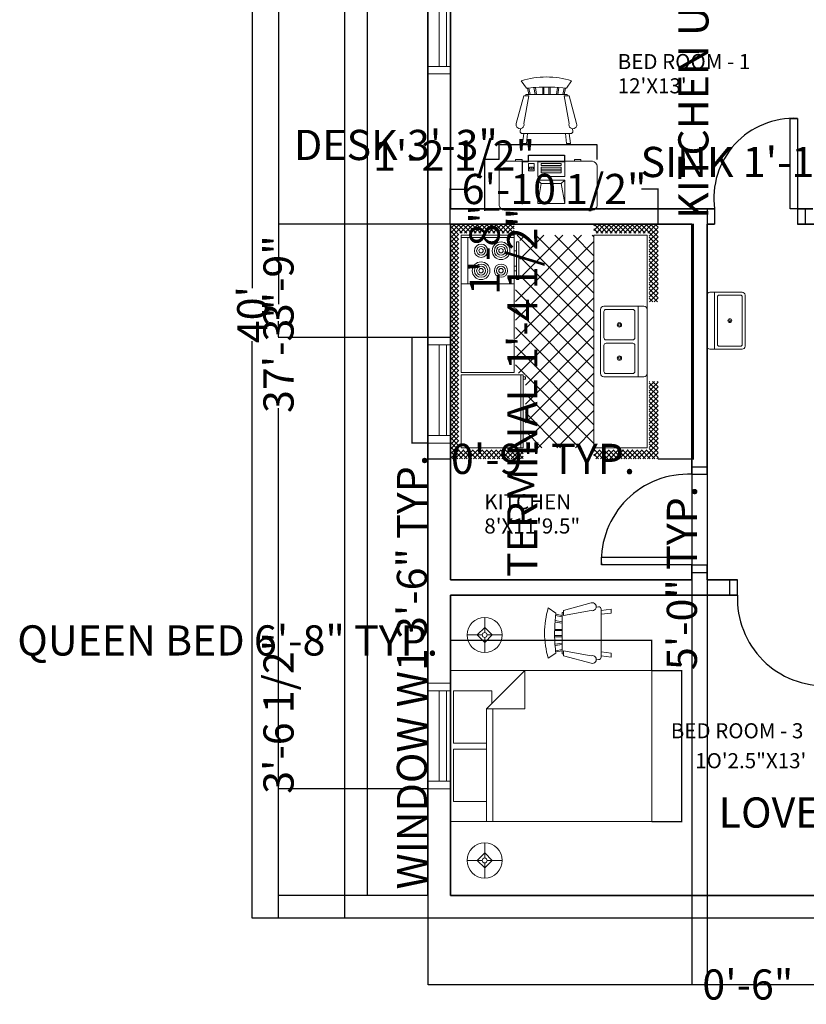
# Model space of a CAD drawing. Units: inches. Extents: x -107 to 531, y -526 to 131.
# Tile 1 of 4: x -107 to 205, y -506 to -114. Entities that reach past the tile are written whole.
import ezdxf

# ---------------------------------------------------------------- set-up
doc = ezdxf.new("R2010")
doc.units = ezdxf.units.IN
doc.header["$MEASUREMENT"] = 0
for name, color, linetype, lineweight in [('A-ANNO-DIMS', 2, 'Continuous', 18), ('A-AREA-IDEN', 7, 'Continuous', 25), ('A-DOOR', 3, 'Continuous', 25), ('A-EQPM', 9, 'Continuous', 18), ('A-FLOR-FIXT', 9, 'Continuous', 18), ('A-FURN', 8, 'Continuous', 18), ('A-GLAZ', 4, 'Continuous', 18), ('A-WALL', 7, 'Continuous', 35), ('C-PROP', 8, 'Continuous', 25)]:
    doc.layers.add(name, color=color, linetype=linetype, lineweight=lineweight)
doc.styles.get("Standard").update_dxf_attribs({"font": 'arial.ttf'})
doc.dimstyles.get("Standard").update_dxf_attribs({"dimtxt": 12, "dimasz": 0.18, "dimexe": 0.18, "dimexo": 0.0625, "dimgap": 0.09, "dimtad": 0, "dimdec": 1, "dimzin": 0, "dimdsep": 46, "dimlunit": 3, "dimtxsty": 'Standard', "dimcen": 0.09, "dimadec": 0, "dimazin": 0, "dimtfac": 1, "dimtdec": 1, "dimtofl": 0, "dimtmove": 0, "dimatfit": 3, "dimfxl": 1, "dimtolj": 1, "dimtzin": 0, "dimarcsym": 0})

# ---------------------------------------------------------------- blocks, each defined once
blk = doc.blocks.new('Bed - Queen')
for p, q in [((0, -80.00003), (0, 0)), ((0, 0), (59.99999, 0)), ((59.99999, 0), (59.99999, -80.00003)), ((7.99999, -1.2), (28.79998, -1.2)), ((7.99999, -14.4), (7.99999, -1.2)), ((28.79998, -1.2), (28.79998, -14.4)), ((31.19999, -1.2), (51.99999, -1.2)), ((31.19999, -14.4), (31.19999, -1.2)), ((51.99999, -1.2), (51.99999, -16.4)), ((0, -14.4), (44.8, -14.4)), ((59.99999, -29.6), (44.8, -14.4)), ((44.8, -14.4), (44.8, -29.6)), ((44.8, -16.8), (0, -16.8)), ((51.99999, -16.4), (46.79936, -16.4)), ((44.8, -29.6), (59.99999, -29.6)), ((59.99999, -80.00003), (0, -80.00003))]:
    blk.add_line(p, q)
blk = doc.blocks.new('Kitchen Layout - 7 x 8 ft')
for p, q in [((-5, 81.32), (2.68, 89)), ((-5, 83.44), (0.56, 89)), ((-5, 85.56), (-1.56, 89)), ((-5, 87.68), (-3.68, 89)), ((1.09, 85), (-2.91, 89)), ((3.21, 85), (-0.79, 89)), ((0.81, 85), (4.81, 89)), ((5.34, 85), (1.34, 89)), ((2.93, 85), (6.93, 89)), ((7.46, 85), (3.46, 89)), ((5.05, 85), (9.05, 89)), ((9.58, 85), (5.58, 89)), ((7.17, 85), (11.17, 89)), ((11.7, 85), (7.7, 89)), ((9.29, 85), (13.29, 89)), ((13.82, 85), (9.82, 89)), ((11.41, 85), (15.41, 89)), ((15.94, 85), (11.94, 89)), ((13.53, 85), (17.53, 89)), ((18.06, 85), (14.06, 89)), ((15.65, 85), (19.65, 89)), ((20.18, 85), (16.18, 89)), ((17.78, 85), (21.78, 89)), ((22.31, 85), (18.31, 89)), ((19.9, 85), (23.9, 89)), ((24.43, 85), (20.43, 89)), ((22.02, 85), (26.02, 89)), ((26.55, 85), (22.55, 89)), ((24.14, 85), (28.14, 89)), ((28.67, 85), (24.67, 89)), ((26.26, 85), (30.26, 89)), ((30.79, 85), (26.79, 89)), ((28.38, 85), (32.38, 89)), ((32.91, 85), (28.91, 89)), ((30.5, 85), (34.5, 89)), ((35.03, 85), (31.03, 89)), ((32.63, 85), (36.63, 89)), ((37.16, 85), (33.16, 89)), ((34.75, 85), (38.75, 89)), ((39.28, 85), (35.28, 89)), ((36.87, 85), (40.87, 89)), ((41.4, 85), (37.4, 89)), ((38.99, 85), (42.99, 89)), ((43.52, 85), (39.52, 89)), ((41.11, 85), (45.11, 89)), ((45.64, 85), (41.64, 89)), ((43.23, 85), (47.23, 89)), ((47.76, 85), (43.76, 89)), ((45.35, 85), (49.35, 89)), ((49.88, 85), (45.88, 89)), ((47.47, 85), (51.47, 89)), ((52, 85), (48, 89)), ((49.6, 85), (53.6, 89)), ((54.13, 85), (50.13, 89)), ((51.72, 85), (55.72, 89)), ((56.25, 85), (52.25, 89)), ((53.84, 85), (57.84, 89)), ((58.37, 85), (54.37, 89)), ((55.96, 85), (59.96, 89)), ((60.49, 85), (56.49, 89)), ((58.08, 85), (62.08, 89)), ((62.61, 85), (58.61, 89)), ((60.2, 85), (64.2, 89)), ((64.73, 85), (60.73, 89)), ((62.32, 85), (66.32, 89)), ((66.85, 85), (62.85, 89)), ((64.45, 85), (68.45, 89)), ((68.97, 85), (64.97, 89)), ((66.57, 85), (70.57, 89)), ((71.1, 85), (67.1, 89)), ((68.69, 85), (72.69, 89)), ((73.22, 85), (69.22, 89)), ((70.81, 85), (74.81, 89)), ((75.34, 85), (71.34, 89)), ((72.93, 85), (76.93, 89)), ((77.46, 85), (73.46, 89)), ((75.05, 85), (79.05, 89)), ((79.58, 85), (75.58, 89)), ((77.17, 85), (81.17, 89)), ((81.7, 85), (77.7, 89)), ((79.29, 85), (83.29, 89)), ((83.82, 85), (79.82, 89)), ((81.42, 85), (85.42, 89)), ((85.95, 85), (81.95, 89)), ((83.54, 85), (87.54, 89)), ((88.07, 85), (84.07, 89)), ((85.66, 85), (89.66, 89)), ((90.19, 85), (86.19, 89)), ((87.78, 85), (91.78, 89)), ((92.31, 85), (88.31, 89)), ((89.9, 85), (93.9, 89)), ((94.43, 85), (90.43, 89)), ((92.02, 85), (96.02, 89)), ((96.55, 85), (92.55, 89)), ((94.14, 85), (98.14, 89)), ((101, 82.67), (94.67, 89)), ((96.27, 85), (100.27, 89)), ((101, 84.79), (96.79, 89)), ((101, 86.92), (98.92, 89)), ((-1, 84.97), (-5, 88.97)), ((-1, 82.85), (-5, 86.85)), ((-1, 80.73), (-5, 84.73)), ((97, 83.61), (101, 87.61)), ((97, 81.49), (101, 85.49)), ((101, 80.55), (97, 84.55)), ((-5, 79.19), (-1, 83.19)), ((-1, 78.61), (-5, 82.61)), ((-5, 77.07), (-1, 81.07)), ((-1, 76.49), (-5, 80.49)), ((34, 84), (96, 84)), ((34, 60), (34, 84)), ((74, 81), (95, 81)), ((96, 84), (96, 60)), ((97, 79.37), (101, 83.37)), ((101, 78.43), (97, 82.43)), ((97, 77.25), (101, 81.25)), ((101, 76.31), (97, 80.31)), ((-5, 74.95), (-1, 78.95)), ((-1, 74.36), (-5, 78.36)), ((-5, 72.83), (-1, 76.83)), ((-1, 72.24), (-5, 76.24)), ((97, 75.13), (101, 79.13)), ((101, 74.19), (97, 78.19)), ((97, 73.01), (101, 77.01)), ((101, 72.07), (97, 76.07)), ((-5, 70.71), (-1, 74.71)), ((-1, 70.12), (-5, 74.12)), ((-5, 68.59), (-1, 72.59)), ((-1, 68), (-5, 72)), ((97, 70.89), (101, 74.89)), ((101, 69.95), (97, 73.95)), ((97, 68.76), (101, 72.76)), ((101, 67.82), (97, 71.82)), ((-5, 66.47), (-1, 70.47)), ((-1, 65.88), (-5, 69.88)), ((-5, 64.35), (-1, 68.35)), ((-1, 63.76), (-5, 67.76)), ((97, 66.64), (101, 70.64)), ((101, 65.7), (97, 69.7)), ((97, 64.52), (101, 68.52)), ((101, 63.58), (97, 67.58)), ((-5, 62.22), (-1, 66.22)), ((-1, 61.64), (-5, 65.64)), ((-5, 60.1), (-1, 64.1)), ((-1, 59.52), (-5, 63.52)), ((97, 62.4), (101, 66.4)), ((101, 61.46), (97, 65.46)), ((97, 60.28), (101, 64.28)), ((100.34, 60), (97, 63.34)), ((-5, 57.98), (-1, 61.98)), ((-1, 57.39), (-5, 61.39)), ((-1.73, 56), (-5, 59.27)), ((-4.86, 56), (-1, 59.86)), ((10.4, 24), (45.9, 59.5)), ((18.88, 24), (54.38, 59.5)), ((27.37, 24), (62.87, 59.5)), ((33.03, 55.11), (37.41, 59.5)), ((67.71, 24), (33.68, 58.04)), ((96, 60), (34, 60)), ((35.85, 24), (71.35, 59.5)), ((76.2, 24), (40.7, 59.5)), ((84.68, 24), (49.18, 59.5)), ((93.17, 24), (57.67, 59.5)), ((61.31, 24), (96, 58.69)), ((96, 29.65), (66.15, 59.5)), ((80, 60), (80, 59)), ((82, 59), (82, 60)), ((87, 59), (87, 60)), ((89, 60), (89, 59)), ((98.22, 60), (97, 61.22)), ((98.84, 60), (101, 62.16)), ((100.96, 60), (101, 60.04)), ((-3.85, 56), (-5, 57.15)), ((-2.74, 56), (-1, 57.74)), ((0, 57), (33, 57)), ((0, 30.57), (24.43, 55)), ((0, 39.06), (15.94, 55)), ((0, 47.54), (7.46, 55)), ((1.91, 24), (32.91, 55)), ((33.77, 24), (2.77, 55)), ((42.26, 24), (11.26, 55)), ((50.74, 24), (19.74, 55)), ((59.23, 24), (28.23, 55)), ((31, 55), (31, 56)), ((32, 55), (31, 55)), ((32, 56), (32, 55)), ((44.34, 24), (77.84, 57.5)), ((52.82, 24), (86.32, 57.5)), ((96, 38.14), (76.64, 57.5)), ((96, 46.63), (85.13, 57.5)), ((96, 55.11), (93.57, 57.54)), ((25.29, 24), (0, 49.29)), ((69.79, 24), (96, 50.21)), ((16.8, 24), (0, 40.8)), ((78.28, 24), (96, 41.72)), ((8.32, 24), (0, 32.32)), ((86.76, 24), (96, 33.24)), ((-5, 21.92), (-2.92, 24)), ((-5, 19.8), (-1, 23.8)), ((-1, 19.21), (-5, 23.21)), ((-1, 21.33), (-3.67, 24)), ((-1, 23.45), (-1.55, 24)), ((0, 24), (96, 24)), ((0, 0), (0, 24)), ((95.25, 24), (96, 24.75)), ((96, 24), (96, 0)), ((97, 22.1), (98.9, 24)), ((97, 19.97), (101, 23.97)), ((101, 19.03), (97, 23.03)), ((101, 21.16), (98.16, 24)), ((101, 23.28), (100.28, 24)), ((-5, 17.68), (-1, 21.68)), ((-1, 17.09), (-5, 21.09)), ((-5, 15.55), (-1, 19.55)), ((-1, 14.97), (-5, 18.97)), ((47.25, 6.5), (47.25, 18.5)), ((48.75, 18.5), (48.75, 6.5)), ((97, 17.85), (101, 21.85)), ((101, 16.91), (97, 20.91)), ((97, 15.73), (101, 19.73)), ((101, 14.79), (97, 18.79)), ((-5, 13.43), (-1, 17.43)), ((-1, 12.85), (-5, 16.85)), ((-5, 11.31), (-1, 15.31)), ((-1, 10.73), (-5, 14.73)), ((97, 13.61), (101, 17.61)), ((101, 12.67), (97, 16.67)), ((97, 11.49), (101, 15.49)), ((101, 10.55), (97, 14.55)), ((97, 9.37), (101, 13.37)), ((-5, 9.19), (-1, 13.19)), ((-1, 8.6), (-5, 12.6)), ((-5, 7.07), (-1, 11.07)), ((-1, 6.48), (-5, 10.48)), ((-5, 4.95), (-1, 8.95)), ((101, 8.43), (97, 12.43)), ((97, 7.25), (101, 11.25)), ((101, 6.31), (97, 10.31)), ((97, 5.12), (101, 9.12)), ((-1, 4.36), (-5, 8.36)), ((-5, 2.83), (-1, 6.83)), ((-1, 2.24), (-5, 6.24)), ((-5, 0.71), (-1, 4.71)), ((101, 4.18), (97, 8.18)), ((97, 3), (101, 7)), ((101, 2.06), (97, 6.06)), ((97, 0.88), (101, 4.88)), ((-1, 0.12), (-5, 4.12)), ((-5, -1.42), (-1, 2.58)), ((2, -5), (-5, 2)), ((-5, -3.54), (-1, 0.46)), ((96, 0), (0, 0)), ((64, 4), (32, 4)), ((93.24, -5), (101, 2.76)), ((95.36, -5), (101, 0.64)), ((101, -0.06), (97, 3.94)), ((101, -2.18), (97, 1.82)), ((-0.12, -5), (-5, -0.12)), ((-2.25, -5), (-5, -2.25)), ((-4.37, -5), (-5, -4.37)), ((-4.34, -5), (-0.34, -1)), ((-2.22, -5), (1.78, -1)), ((-0.1, -5), (3.9, -1)), ((4.12, -5), (0.12, -1)), ((2.02, -5), (6.02, -1)), ((6.24, -5), (2.24, -1)), ((4.14, -5), (8.14, -1)), ((8.36, -5), (4.36, -1)), ((6.27, -5), (10.27, -1)), ((10.48, -5), (6.48, -1)), ((8.39, -5), (12.39, -1)), ((12.6, -5), (8.6, -1)), ((10.51, -5), (14.51, -1)), ((14.73, -5), (10.73, -1)), ((12.63, -5), (16.63, -1)), ((16.85, -5), (12.85, -1)), ((14.75, -5), (18.75, -1)), ((18.97, -5), (14.97, -1)), ((16.87, -5), (20.87, -1)), ((21.09, -5), (17.09, -1)), ((18.99, -5), (22.99, -1)), ((23.21, -5), (19.21, -1)), ((21.11, -5), (25.11, -1)), ((25.33, -5), (21.33, -1)), ((23.24, -5), (27.24, -1)), ((27.45, -5), (23.45, -1)), ((25.36, -5), (29.36, -1)), ((29.57, -5), (25.57, -1)), ((27.48, -5), (30, -2.48)), ((30, -3.3), (27.7, -1)), ((30, -1.18), (29.82, -1)), ((66, -2.54), (67.54, -1)), ((66, -4.66), (69.66, -1)), ((69.88, -5), (66, -1.12)), ((67.76, -5), (66, -3.24)), ((67.78, -5), (71.78, -1)), ((72, -5), (68, -1)), ((69.9, -5), (73.9, -1)), ((74.12, -5), (70.12, -1)), ((72.03, -5), (76.03, -1)), ((76.24, -5), (72.24, -1)), ((74.15, -5), (78.15, -1)), ((78.36, -5), (74.36, -1)), ((76.27, -5), (80.27, -1)), ((80.49, -5), (76.49, -1)), ((78.39, -5), (82.39, -1)), ((82.61, -5), (78.61, -1)), ((80.51, -5), (84.51, -1)), ((84.73, -5), (80.73, -1)), ((82.63, -5), (86.63, -1)), ((86.85, -5), (82.85, -1)), ((84.75, -5), (88.75, -1)), ((88.97, -5), (84.97, -1)), ((86.88, -5), (90.88, -1)), ((91.09, -5), (87.09, -1)), ((89, -5), (93, -1)), ((93.21, -5), (89.21, -1)), ((91.12, -5), (95.12, -1)), ((95.34, -5), (91.34, -1)), ((97.46, -5), (93.46, -1)), ((99.58, -5), (95.58, -1)), ((101, -4.3), (97, -0.3)), ((97.48, -5), (101, -1.48)), ((99.6, -5), (101, -3.6)), ((29.6, -5), (30, -4.6))]:
    blk.add_line(p, q)
for points in [[(0, 56), (0, 84), (33, 84), (33, 56)], [(74, 60), (74, 84), (95, 84), (95, 60)], [(76, 58), (76, 59), (93, 59), (93, 58)]]:
    blk.add_lwpolyline(points, close=True)
for points in [[(32, 1.5), (32, 19.5)], [(33.5, 21), (62.5, 21)], [(33.5, 6.5), (33.5, 18.5)], [(34.5, 19.5), (46.25, 19.5)], [(49.75, 19.5), (61.5, 19.5)], [(62.5, 18.5), (62.5, 6.5)], [(64, 19.5), (64, 1.5)], [(46.25, 5.5), (34.5, 5.5)], [(61.5, 5.5), (49.75, 5.5)], [(62.5, 0), (33.5, 0)]]:
    blk.add_lwpolyline(points)
for centre, radius in [((80, 75), 4), ((80, 75), 3), ((80, 75), 2), ((80, 75), 1), ((89, 75), 3), ((89, 75), 2), ((89, 75), 1), ((80, 66), 3), ((80, 66), 2), ((80, 66), 1), ((89, 66), 4), ((89, 66), 3), ((89, 66), 2), ((89, 66), 1), ((40.5, 12.5), 1), ((55.5, 12.5), 1), ((40.5, 12.5), 0.5), ((55.5, 12.5), 0.5)]:
    blk.add_circle(centre, radius)
for centre, radius, start, end in [((33.5, 19.5), 1.5, 90, 180), ((34.5, 18.5), 1, 90, 180), ((46.25, 18.5), 1, 0, 90), ((49.75, 18.5), 1, 90, 180), ((61.5, 18.5), 1, 0, 90), ((62.5, 19.5), 1.5, 0, 90), ((34.5, 6.5), 1, 180, 270), ((46.25, 6.5), 1, 270, 0), ((49.75, 6.5), 1, 180, 270), ((61.5, 6.5), 1, 270, 0), ((33.5, 1.5), 1.5, 180, 270), ((62.5, 1.5), 1.5, 270, 0)]:
    blk.add_arc(centre, radius, start, end)
blk = doc.blocks.new('Lamp - Table')
for p, q in [((0, 7), (0, 1)), ((-1, 0), (-7, 0)), ((0, 3), (-3, 0)), ((-3, 0), (0, -3)), ((3, 0), (0, 3)), ((0, -3), (3, 0)), ((1, 0), (7, 0)), ((0, -1), (0, -7))]:
    blk.add_line(p, q)
for radius in [7, 1]:
    blk.add_circle((0, 0), radius)
blk = doc.blocks.new('Sink-single - 30 in top')
blk.add_line((-15, -3.999996), (15, -3.999996))
for points in [[(-13.5, 0), (13.5, 0)], [(-15, -18.499996), (-15, -1.5)], [(15, -1.5), (15, -18.499996)], [(-13.5, -17.499996), (-13.5, -6.499996)], [(-12.5, -5.499996), (12.5, -5.499996)], [(13.5, -6.499996), (13.5, -17.499996)], [(13.5, -19.999996), (-13.5, -19.999996)], [(12.5, -18.499996), (-12.5, -18.499996)]]:
    blk.add_lwpolyline(points)
for radius in [1, 0.5]:
    blk.add_circle((0, -11.999996), radius)
for centre, radius, start, end in [((-13.5, -1.5), 1.5, 90, 180), ((13.5, -1.5), 1.5, 0, 90), ((-12.5, -6.499996), 1, 90, 180), ((12.5, -6.499996), 1, 0, 90), ((-13.5, -18.499996), 1.5, 180, 270), ((-12.5, -17.499996), 1, 180, 270), ((12.5, -17.499996), 1, 270, 0), ((13.5, -18.499996), 1.5, 270, 0)]:
    blk.add_arc(centre, radius, start, end)
blk = doc.blocks.new('Chair - Rocking')
for p, q in [((-8, -4.5), (-10, -1.5)), ((8, -4.5), (10, -1.5)), ((-9, -7.5), (-12, -18.49999)), ((-7, -7.5), (-9, -7.5)), ((-9, -18.49999), (-7, -7.5)), ((-8.23428, -6.99939), (-8.3093, -7.47958)), ((-8.23041, -7), (8.23915, -7)), ((-7.5, -4.5), (-7, -7)), ((-6.5, -7), (-7.02225, -4.43)), ((-4.5, -7), (-4.96674, -4.19951)), ((-4, -7), (-4.40532, -4.16272)), ((-1.5, -4.05012), (-1.5, -7)), ((-1, -7), (-1, -4.05012)), ((1, -7), (1, -4.04655)), ((1.5, -4.05012), (1.5, -7)), ((4, -7), (4.40187, -4.18694)), ((4.5, -7), (4.96761, -4.19437)), ((6.5, -7), (7, -4.4057)), ((7.5, -4.5), (7, -7)), ((7, -7.5), (9, -7.5)), ((9, -18.49999), (7, -7.5)), ((8.31071, -7.48854), (8.23449, -7.00073)), ((9, -7.5), (12, -18.49999)), ((-10.36644, -20.64523), (-10.5, -21.49999)), ((-9, -22.49999), (-9.5, -26.49999)), ((0, -22.49999), (-9.5, -22.49999)), ((-8, -26.49999), (-7.5, -22.49999)), ((0, -22.49999), (9.5, -22.49999)), ((8, -26.49999), (7.5, -22.49999)), ((9, -22.49999), (9.5, -26.49999)), ((10.5, -21.49999), (10.3575, -20.58798)), ((-9.5, -26.49999), (-8, -26.49999)), ((9.5, -26.49999), (8, -26.49999))]:
    blk.add_line(p, q)
for centre, radius, start, end in [((0, -34.08333), 34.08333, 72.93847, 107.0615), ((0, -68.25004), 64.25, 93.92211, 97.15267), ((0, -68.25004), 64.25, 82.84733, 93.92211), ((-10.5, -18.99999), 1.58114, 161.5651, 18.43495), ((10.5, -18.99999), 1.58114, 161.5651, 18.43495), ((-9.5, -21.49999), 1, 180, 270), ((9.5, -21.49999), 1, 270, 0)]:
    blk.add_arc(centre, radius, start, end)
blk = doc.blocks.new('Desk - 30 x 60 in.')
for p, q in [((-26.999995, 0), (26.999995, 0)), ((-29.999995, -27), (-29.999995, -3)), ((29.999995, -3), (29.999995, -27)), ((26.999995, -30), (-26.999995, -30)), ((-20.000005, -30), (-20.000005, -31)), ((-16.000005, -31), (-16.000005, -30)), ((15.999995, -31), (15.999995, -30)), ((19.999995, -30), (19.999995, -31)), ((-20.000005, -31), (-16.000005, -31)), ((19.999995, -31), (15.999995, -31))]:
    blk.add_line(p, q)
for centre, start, end in [((-26.499995, -3.5), 98.1301, 171.8699), ((26.499995, -3.5), 8.130102, 81.8699), ((-26.499995, -26.5), 188.1301, 261.8699), ((26.499995, -26.5), 278.1301, 351.8699)]:
    blk.add_arc(centre, 3.535534, start, end)
blk = doc.blocks.new('Computer Terminal')
for p, q in [((-10, 11.5), (5, 11.5)), ((-8, 0.5), (-10, 11.5)), ((-10, -1.5), (-10, 11.5)), ((5, 11.5), (3, 0.5)), ((5, 11.5), (5, -1.5)), ((-10, -1.5), (-8, 0.5)), ((3, 0.5), (-8, 0.5)), ((3, 0.5), (5, -1.5)), ((5, -1.5), (-10, -1.5)), ((-10, -11.5), (-10, -3.5)), ((-10, -3.5), (5, -3.5)), ((5, -3.5), (5, -11.5)), ((-8, -5.5), (-8, -8.5)), ((3, -5.5), (-8, -5.5)), ((3, -6.5), (-8, -6.5)), ((-8, -7.5), (3, -7.5)), ((-8, -8.5), (3, -8.5)), ((-8, -9.5), (-8, -10.5)), ((3, -9.5), (-8, -9.5)), ((-8, -10.5), (3, -10.5)), ((3, -8.5), (3, -5.5)), ((3, -10.5), (3, -9.5)), ((10, -6.5), (7, -6.5)), ((7, -6.5), (7, -10.5)), ((7, -10.5), (10, -10.5)), ((9.5, -7.5), (7.5, -7.5)), ((7.5, -7.5), (7.5, -8.5)), ((7.5, -8.5), (9.5, -8.5)), ((8.5, -7.5), (8.5, -8.5)), ((9.5, -8.5), (9.5, -7.5)), ((10, -10.5), (10, -6.5)), ((5, -11.5), (-10, -11.5))]:
    blk.add_line(p, q)
blk = doc.blocks.new('*D18')
at = {"layer": 'A-ANNO-DIMS', "color": 0, "lineweight": -2, "transparency": 16777216}
for p, q in [((21.89, 8.64), (-15.01, 8.64)), ((-14.83, 8.46), (-14.83, -220.85)), ((-14.83, -471.18), (-14.83, -241.88)), ((21.89, -471.36), (-15.01, -471.36))]:
    blk.add_line(p, q, dxfattribs=at)
at = {"layer": 'A-ANNO-DIMS', "color": 0, "transparency": 16777216}
for points in [[(-14.86, 8.46), (-14.8, 8.46), (-14.83, 8.64)], [(-14.86, -471.18), (-14.8, -471.18), (-14.83, -471.36)]]:
    blk.add_solid(points, dxfattribs=at)
at = {"layer": 'Defpoints', "color": 0, "transparency": 16777216}
for p in [(21.95, 8.64), (-14.83, -471.36), (21.95, -471.36)]:
    blk.add_point(p, dxfattribs=at)
at = {"layer": 'A-ANNO-DIMS', "color": 0, "transparency": 16777216, "insert": (-14.83, -231.36), "char_height": 12, "attachment_point": 5, "rotation": 90}
blk.add_mtext("\\A1;40'", dxfattribs=at)
blk = doc.blocks.new('WIN-36')
for p, q in [((0, 0), (0, 9)), ((3, 0), (3, 9)), ((3, 9), (39, 9)), ((39, 9), (39, 0)), ((42, 9), (42, 0)), ((39, 7.5), (3, 7.5)), ((39, 4.5), (3, 4.5)), ((39, 0), (3, 0))]:
    blk.add_line(p, q)
blk = doc.blocks.new('DOOR-36-SWING')
for p, q in [((36.03, 42), (42.03, 42)), ((36.03, 39), (42.03, 39)), ((36.03, 3), (42.03, 3)), ((36.03, 0), (42.03, 0))]:
    blk.add_line(p, q)
blk.add_lwpolyline([(36.03, 3), (0.03, 3), (0.03, 6), (36.03, 6)], close=True)
blk.add_arc((34.53, 4.5), 34.53, 87.5104, 182.4896)
blk = doc.blocks.new('*D23')
at = {"layer": 'A-ANNO-DIMS', "color": 0, "lineweight": -2, "transparency": 16777216}
for p, q in [((54.89, -240.42), (48.47, -240.42)), ((48.65, -240.6), (48.65, -282.24)), ((54.89, -282.42), (48.47, -282.42)), ((48.65, -282.42), (48.65, -282.6))]:
    blk.add_line(p, q, dxfattribs=at)
at = {"layer": 'A-ANNO-DIMS', "color": 0, "transparency": 16777216}
for points in [[(48.62, -240.6), (48.68, -240.6), (48.65, -240.42)], [(48.62, -282.24), (48.68, -282.24), (48.65, -282.42)]]:
    blk.add_solid(points, dxfattribs=at)
at = {"layer": 'Defpoints', "color": 0, "transparency": 16777216}
for p in [(54.95, -240.42), (48.65, -282.42), (54.95, -282.42)]:
    blk.add_point(p, dxfattribs=at)
at = {"layer": 'A-ANNO-DIMS', "color": 0, "transparency": 16777216, "insert": (48.65, -373.51), "char_height": 12, "attachment_point": 5, "rotation": 90}
blk.add_mtext('\\A1;WINDOW W1 3\'-6" TYP.', dxfattribs=at)
blk = doc.blocks.new('*D24')
at = {"layer": 'A-ANNO-DIMS', "color": 0, "lineweight": -2, "transparency": 16777216}
for p, q in [((54.95, -282.48), (54.95, -288.9)), ((63.95, -282.48), (63.95, -288.9)), ((55.13, -288.72), (63.77, -288.72)), ((63.95, -288.72), (64.13, -288.72))]:
    blk.add_line(p, q, dxfattribs=at)
at = {"layer": 'A-ANNO-DIMS', "color": 0, "transparency": 16777216}
for points in [[(55.13, -288.69), (55.13, -288.75), (54.95, -288.72)], [(63.77, -288.69), (63.77, -288.75), (63.95, -288.72)]]:
    blk.add_solid(points, dxfattribs=at)
at = {"layer": 'Defpoints', "color": 0, "transparency": 16777216}
for p in [(54.95, -282.42), (63.95, -282.42), (63.95, -288.72)]:
    blk.add_point(p, dxfattribs=at)
at = {"layer": 'A-ANNO-DIMS', "color": 0, "transparency": 16777216, "insert": (100.79, -288.72), "char_height": 12, "attachment_point": 5}
blk.add_mtext('\\A1;0\'-9" TYP.', dxfattribs=at)
blk = doc.blocks.new('*D31')
at = {"layer": 'A-ANNO-DIMS', "color": 0, "lineweight": -2, "transparency": 16777216}
for p, q in [((63.95, -360.91), (63.77, -360.91)), ((63.95, -372.85), (63.95, -360.73)), ((143.77, -360.91), (64.13, -360.91)), ((143.95, -372.85), (143.95, -360.73))]:
    blk.add_line(p, q, dxfattribs=at)
at = {"layer": 'A-ANNO-DIMS', "color": 0, "transparency": 16777216}
for points in [[(64.13, -360.88), (64.13, -360.94), (63.95, -360.91)], [(143.77, -360.88), (143.77, -360.94), (143.95, -360.91)]]:
    blk.add_solid(points, dxfattribs=at)
at = {"layer": 'Defpoints', "color": 0, "transparency": 16777216}
for p in [(63.95, -360.91), (63.95, -372.91), (143.95, -372.91)]:
    blk.add_point(p, dxfattribs=at)
at = {"layer": 'A-ANNO-DIMS', "color": 0, "transparency": 16777216, "insert": (-24.58, -360.91), "char_height": 12, "attachment_point": 5}
blk.add_mtext('\\A1;QUEEN BED 6\'-8" TYP.', dxfattribs=at)
blk = doc.blocks.new('*D32')
at = {"layer": 'A-ANNO-DIMS', "color": 0, "lineweight": -2, "transparency": 16777216}
for p, q in [((144.01, -372.91), (156.13, -372.91)), ((155.95, -372.91), (155.95, -372.73)), ((155.95, -432.73), (155.95, -373.09)), ((144.01, -432.91), (156.13, -432.91))]:
    blk.add_line(p, q, dxfattribs=at)
at = {"layer": 'A-ANNO-DIMS', "color": 0, "transparency": 16777216}
for points in [[(155.92, -373.09), (155.98, -373.09), (155.95, -372.91)], [(155.92, -432.73), (155.98, -432.73), (155.95, -432.91)]]:
    blk.add_solid(points, dxfattribs=at)
at = {"layer": 'Defpoints', "color": 0, "transparency": 16777216}
for p in [(143.95, -372.91), (155.95, -372.91), (143.95, -432.91)]:
    blk.add_point(p, dxfattribs=at)
at = {"layer": 'A-ANNO-DIMS', "color": 0, "transparency": 16777216, "insert": (155.95, -336.07), "char_height": 12, "attachment_point": 5, "rotation": 90}
blk.add_mtext('\\A1;5\'-0" TYP.', dxfattribs=at)
blk = doc.blocks.new('*D41')
at = {"layer": 'A-ANNO-DIMS', "color": 0, "lineweight": -2, "transparency": 16777216}
for p, q in [((225.21, -170.68), (225.03, -170.68)), ((225.21, -174.05), (225.21, -170.5)), ((247.92, -170.68), (225.39, -170.68)), ((248.1, -174.05), (248.1, -170.5))]:
    blk.add_line(p, q, dxfattribs=at)
at = {"layer": 'A-ANNO-DIMS', "color": 0, "transparency": 16777216}
for points in [[(225.39, -170.65), (225.39, -170.71), (225.21, -170.68)], [(247.92, -170.65), (247.92, -170.71), (248.1, -170.68)]]:
    blk.add_solid(points, dxfattribs=at)
at = {"layer": 'Defpoints', "color": 0, "transparency": 16777216}
for p in [(225.21, -170.68), (225.21, -174.11), (248.1, -174.11)]:
    blk.add_point(p, dxfattribs=at)
at = {"layer": 'A-ANNO-DIMS', "color": 0, "transparency": 16777216, "insert": (182.47, -170.68), "char_height": 12, "attachment_point": 5}
blk.add_mtext('\\A1;SINK 1\'-11"', dxfattribs=at)
blk = doc.blocks.new('*D42')
at = {"layer": 'A-ANNO-DIMS', "color": 0, "lineweight": -2, "transparency": 16777216}
for p, q in [((225.15, -174.11), (221.6, -174.11)), ((221.78, -174.29), (221.78, -189.18)), ((225.15, -189.36), (221.6, -189.36)), ((221.78, -189.36), (221.78, -189.54))]:
    blk.add_line(p, q, dxfattribs=at)
at = {"layer": 'A-ANNO-DIMS', "color": 0, "transparency": 16777216}
for points in [[(221.75, -174.29), (221.81, -174.29), (221.78, -174.11)], [(221.75, -189.18), (221.81, -189.18), (221.78, -189.36)]]:
    blk.add_solid(points, dxfattribs=at)
at = {"layer": 'Defpoints', "color": 0, "transparency": 16777216}
for p in [(225.21, -174.11), (221.78, -189.36), (225.21, -189.36)]:
    blk.add_point(p, dxfattribs=at)
at = {"layer": 'A-ANNO-DIMS', "color": 0, "transparency": 16777216, "insert": (221.78, -219), "char_height": 12, "attachment_point": 5, "rotation": 90}
blk.add_mtext('\\A1;1\'-3 1/2"', dxfattribs=at)
blk = doc.blocks.new('*D47')
at = {"layer": 'A-ANNO-DIMS', "color": 0, "lineweight": -2, "transparency": 16777216}
for p, q in [((320.77, -429.33), (320.59, -429.33)), ((320.77, -435.18), (320.77, -429.15)), ((359.96, -429.33), (320.95, -429.33)), ((360.14, -435.18), (360.14, -429.15))]:
    blk.add_line(p, q, dxfattribs=at)
at = {"layer": 'A-ANNO-DIMS', "color": 0, "transparency": 16777216}
for points in [[(320.95, -429.3), (320.95, -429.36), (320.77, -429.33)], [(359.96, -429.3), (359.96, -429.36), (360.14, -429.33)]]:
    blk.add_solid(points, dxfattribs=at)
at = {"layer": 'Defpoints', "color": 0, "transparency": 16777216}
for p in [(320.77, -429.33), (320.77, -435.24), (360.14, -435.24)]:
    blk.add_point(p, dxfattribs=at)
at = {"layer": 'A-ANNO-DIMS', "color": 0, "transparency": 16777216, "insert": (244.25, -429.33), "char_height": 12, "attachment_point": 5}
blk.add_mtext('\\A1;LOVESEAT 3\'-3 1/2"', dxfattribs=at)
blk = doc.blocks.new('*D51')
at = {"layer": 'A-ANNO-DIMS', "color": 0, "lineweight": -2, "transparency": 16777216}
for p, q in [((146.59, -195.42), (160.7, -195.42)), ((160.52, -195.42), (160.52, -195.24)), ((160.52, -288.52), (160.52, -195.6)), ((146.59, -288.7), (160.7, -288.7))]:
    blk.add_line(p, q, dxfattribs=at)
at = {"layer": 'A-ANNO-DIMS', "color": 0, "transparency": 16777216}
for points in [[(160.49, -195.6), (160.55, -195.6), (160.52, -195.42)], [(160.49, -288.52), (160.55, -288.52), (160.52, -288.7)]]:
    blk.add_solid(points, dxfattribs=at)
at = {"layer": 'Defpoints', "color": 0, "transparency": 16777216}
for p in [(146.53, -195.42), (160.52, -195.42), (146.53, -288.7)]:
    blk.add_point(p, dxfattribs=at)
at = {"layer": 'A-ANNO-DIMS', "color": 0, "transparency": 16777216, "insert": (160.52, -98.9), "char_height": 12, "attachment_point": 5, "rotation": 90}
blk.add_mtext('\\A1;KITCHEN UNITS 7\'-9 1/2"', dxfattribs=at)
blk = doc.blocks.new('*D52')
at = {"layer": 'A-ANNO-DIMS', "color": 0, "lineweight": -2, "transparency": 16777216}
for p, q in [((63.81, -195.36), (63.81, -181.25)), ((63.99, -181.43), (70.45, -181.43)), ((146.35, -181.43), (139.88, -181.43)), ((146.53, -195.36), (146.53, -181.25))]:
    blk.add_line(p, q, dxfattribs=at)
at = {"layer": 'A-ANNO-DIMS', "color": 0, "transparency": 16777216}
for points in [[(63.99, -181.4), (63.99, -181.46), (63.81, -181.43)], [(146.35, -181.4), (146.35, -181.46), (146.53, -181.43)]]:
    blk.add_solid(points, dxfattribs=at)
at = {"layer": 'Defpoints', "color": 0, "transparency": 16777216}
for p in [(63.81, -181.43), (63.81, -195.42), (146.53, -195.42)]:
    blk.add_point(p, dxfattribs=at)
at = {"layer": 'A-ANNO-DIMS', "color": 0, "transparency": 16777216, "insert": (105.17, -181.43), "char_height": 12, "attachment_point": 5}
blk.add_mtext('\\A1;6\'-10 1/2"', dxfattribs=at)
blk = doc.blocks.new('*D55')
at = {"layer": 'A-ANNO-DIMS', "color": 0, "lineweight": -2, "transparency": 16777216}
for p, q in [((83.37, -163.91), (83.19, -163.91)), ((83.37, -169.69), (83.37, -163.73)), ((122.13, -163.91), (83.55, -163.91)), ((122.31, -169.69), (122.31, -163.73))]:
    blk.add_line(p, q, dxfattribs=at)
at = {"layer": 'A-ANNO-DIMS', "color": 0, "transparency": 16777216}
for points in [[(83.55, -163.88), (83.55, -163.94), (83.37, -163.91)], [(122.13, -163.88), (122.13, -163.94), (122.31, -163.91)]]:
    blk.add_solid(points, dxfattribs=at)
at = {"layer": 'Defpoints', "color": 0, "transparency": 16777216}
for p in [(83.37, -163.91), (83.37, -169.75), (122.31, -169.75)]:
    blk.add_point(p, dxfattribs=at)
at = {"layer": 'A-ANNO-DIMS', "color": 0, "transparency": 16777216, "insert": (42.29, -163.91), "char_height": 12, "attachment_point": 5}
blk.add_mtext('\\A1;DESK 3\'-3"', dxfattribs=at)
blk = doc.blocks.new('*D56')
at = {"layer": 'A-ANNO-DIMS', "color": 0, "lineweight": -2, "transparency": 16777216}
for p, q in [((83.3, -169.75), (77.35, -169.75)), ((77.53, -169.93), (77.53, -189.69)), ((83.3, -189.87), (77.35, -189.87)), ((77.53, -189.87), (77.53, -190.05))]:
    blk.add_line(p, q, dxfattribs=at)
at = {"layer": 'A-ANNO-DIMS', "color": 0, "transparency": 16777216}
for points in [[(77.5, -169.93), (77.56, -169.93), (77.53, -169.75)], [(77.5, -189.69), (77.56, -189.69), (77.53, -189.87)]]:
    blk.add_solid(points, dxfattribs=at)
at = {"layer": 'Defpoints', "color": 0, "transparency": 16777216}
for p in [(83.37, -169.75), (77.53, -189.87), (83.37, -189.87)]:
    blk.add_point(p, dxfattribs=at)
at = {"layer": 'A-ANNO-DIMS', "color": 0, "transparency": 16777216, "insert": (77.53, -205.53), "char_height": 12, "attachment_point": 5, "rotation": 90}
blk.add_mtext('\\A1;1\'-8"', dxfattribs=at)
blk = doc.blocks.new('*D57')
at = {"layer": 'A-ANNO-DIMS', "color": 0, "lineweight": -2, "transparency": 16777216}
for p, q in [((94.95, -170.63), (92.34, -170.63)), ((92.52, -170.81), (92.52, -187.07)), ((94.95, -187.25), (92.34, -187.25)), ((92.52, -187.25), (92.52, -187.43))]:
    blk.add_line(p, q, dxfattribs=at)
at = {"layer": 'A-ANNO-DIMS', "color": 0, "transparency": 16777216}
for points in [[(92.49, -170.81), (92.55, -170.81), (92.52, -170.63)], [(92.49, -187.07), (92.55, -187.07), (92.52, -187.25)]]:
    blk.add_solid(points, dxfattribs=at)
at = {"layer": 'Defpoints', "color": 0, "transparency": 16777216}
for p in [(95.02, -170.63), (92.52, -187.25), (95.02, -187.25)]:
    blk.add_point(p, dxfattribs=at)
at = {"layer": 'A-ANNO-DIMS', "color": 0, "transparency": 16777216, "insert": (92.52, -262.31), "char_height": 12, "attachment_point": 5, "rotation": 90}
blk.add_mtext('\\A1;TERMINAL 1\'-4 1/2"', dxfattribs=at)
blk = doc.blocks.new('*D58')
at = {"layer": 'A-ANNO-DIMS', "color": 0, "lineweight": -2, "transparency": 16777216}
for p, q in [((95.02, -168.14), (94.84, -168.14)), ((95.02, -170.57), (95.02, -167.96)), ((109.29, -168.14), (95.2, -168.14)), ((109.47, -170.57), (109.47, -167.96))]:
    blk.add_line(p, q, dxfattribs=at)
at = {"layer": 'A-ANNO-DIMS', "color": 0, "transparency": 16777216}
for points in [[(95.2, -168.11), (95.2, -168.17), (95.02, -168.14)], [(109.29, -168.11), (109.29, -168.17), (109.47, -168.14)]]:
    blk.add_solid(points, dxfattribs=at)
at = {"layer": 'Defpoints', "color": 0, "transparency": 16777216}
for p in [(95.02, -168.14), (95.02, -170.63), (109.47, -170.63)]:
    blk.add_point(p, dxfattribs=at)
at = {"layer": 'A-ANNO-DIMS', "color": 0, "transparency": 16777216, "insert": (65.38, -168.14), "char_height": 12, "attachment_point": 5}
blk.add_mtext('\\A1;1\'-2 1/2"', dxfattribs=at)
blk = doc.blocks.new('*D59')
at = {"layer": 'A-ANNO-DIMS', "color": 0, "lineweight": -2, "transparency": 16777216}
for p, q in [((54.95, -462.42), (54.95, -497.89)), ((444.95, -462.42), (444.95, -497.89)), ((55.13, -497.71), (229.25, -497.71)), ((444.77, -497.71), (270.65, -497.71))]:
    blk.add_line(p, q, dxfattribs=at)
at = {"layer": 'A-ANNO-DIMS', "color": 0, "transparency": 16777216}
for points in [[(55.13, -497.68), (55.13, -497.74), (54.95, -497.71)], [(444.77, -497.68), (444.77, -497.74), (444.95, -497.71)]]:
    blk.add_solid(points, dxfattribs=at)
at = {"layer": 'Defpoints', "color": 0, "transparency": 16777216}
for p in [(54.95, -462.36), (444.95, -462.36), (444.95, -497.71)]:
    blk.add_point(p, dxfattribs=at)
at = {"layer": 'A-ANNO-DIMS', "color": 0, "transparency": 16777216, "insert": (249.95, -497.71), "char_height": 12, "attachment_point": 5}
blk.add_mtext('\\A1;32\'-6"', dxfattribs=at)
blk = doc.blocks.new('*D60')
at = {"layer": 'A-ANNO-DIMS', "color": 0, "lineweight": -2, "transparency": 16777216}
for p, q in [((54.89, -24.36), (-4.58, -24.36)), ((-4.4, -24.54), (-4.4, -227.16)), ((-4.4, -471.18), (-4.4, -268.56)), ((21.89, -471.36), (-4.58, -471.36))]:
    blk.add_line(p, q, dxfattribs=at)
at = {"layer": 'A-ANNO-DIMS', "color": 0, "transparency": 16777216}
for points in [[(-4.43, -24.54), (-4.37, -24.54), (-4.4, -24.36)], [(-4.43, -471.18), (-4.37, -471.18), (-4.4, -471.36)]]:
    blk.add_solid(points, dxfattribs=at)
at = {"layer": 'Defpoints', "color": 0, "transparency": 16777216}
for p in [(54.95, -24.36), (-4.4, -471.36), (21.95, -471.36)]:
    blk.add_point(p, dxfattribs=at)
at = {"layer": 'A-ANNO-DIMS', "color": 0, "transparency": 16777216, "insert": (-4.4, -247.86), "char_height": 12, "attachment_point": 5, "rotation": 90}
blk.add_mtext('\\A1;37\'-3"', dxfattribs=at)
blk = doc.blocks.new('*D71')
at = {"layer": 'A-ANNO-DIMS', "color": 0, "lineweight": -2, "transparency": 16777216}
for p, q in [((54.89, -419.89), (-4.58, -419.89)), ((-4.4, -419.89), (-4.4, -419.71)), ((-4.4, -462.18), (-4.4, -420.07)), ((54.89, -462.36), (-4.58, -462.36))]:
    blk.add_line(p, q, dxfattribs=at)
at = {"layer": 'A-ANNO-DIMS', "color": 0, "transparency": 16777216}
for points in [[(-4.43, -420.07), (-4.37, -420.07), (-4.4, -419.89)], [(-4.43, -462.18), (-4.37, -462.18), (-4.4, -462.36)]]:
    blk.add_solid(points, dxfattribs=at)
at = {"layer": 'Defpoints', "color": 0, "transparency": 16777216}
for p in [(-4.4, -419.89), (54.95, -419.89), (54.95, -462.36)]:
    blk.add_point(p, dxfattribs=at)
at = {"layer": 'A-ANNO-DIMS', "color": 0, "transparency": 16777216, "insert": (-4.4, -389.69), "char_height": 12, "attachment_point": 5, "rotation": 90}
blk.add_mtext('\\A1;3\'-6 1/2"', dxfattribs=at)
blk = doc.blocks.new('*D72')
at = {"layer": 'A-ANNO-DIMS', "color": 0, "lineweight": -2, "transparency": 16777216}
for p, q in [((63.89, -195.36), (-4.58, -195.36)), ((-4.4, -195.54), (-4.4, -201.85)), ((-4.4, -240.24), (-4.4, -233.93)), ((63.89, -240.42), (-4.58, -240.42))]:
    blk.add_line(p, q, dxfattribs=at)
at = {"layer": 'A-ANNO-DIMS', "color": 0, "transparency": 16777216}
for points in [[(-4.43, -195.54), (-4.37, -195.54), (-4.4, -195.36)], [(-4.43, -240.24), (-4.37, -240.24), (-4.4, -240.42)]]:
    blk.add_solid(points, dxfattribs=at)
at = {"layer": 'Defpoints', "color": 0, "transparency": 16777216}
for p in [(63.95, -195.36), (-4.4, -240.42), (63.95, -240.42)]:
    blk.add_point(p, dxfattribs=at)
at = {"layer": 'A-ANNO-DIMS', "color": 0, "transparency": 16777216, "insert": (-4.4, -217.89), "char_height": 12, "attachment_point": 5, "rotation": 90}
blk.add_mtext('\\A1;3\'-9"', dxfattribs=at)
blk = doc.blocks.new('*D75')
at = {"layer": 'A-ANNO-DIMS', "color": 0, "lineweight": -2, "transparency": 16777216}
for p, q in [((159.95, -195.42), (159.95, -497.89)), ((165.95, -195.42), (165.95, -497.89)), ((160.13, -497.71), (165.77, -497.71)), ((165.95, -497.71), (166.13, -497.71))]:
    blk.add_line(p, q, dxfattribs=at)
at = {"layer": 'A-ANNO-DIMS', "color": 0, "transparency": 16777216}
for points in [[(160.13, -497.68), (160.13, -497.74), (159.95, -497.71)], [(165.77, -497.68), (165.77, -497.74), (165.95, -497.71)]]:
    blk.add_solid(points, dxfattribs=at)
at = {"layer": 'Defpoints', "color": 0, "transparency": 16777216}
for p in [(159.95, -195.36), (165.95, -195.36), (165.95, -497.71)]:
    blk.add_point(p, dxfattribs=at)
at = {"layer": 'A-ANNO-DIMS', "color": 0, "transparency": 16777216, "insert": (182.17, -497.71), "char_height": 12, "attachment_point": 5}
blk.add_mtext('\\A1;0\'-6"', dxfattribs=at)

msp = doc.modelspace()

# ---------------------------------------------------------------- linework, layer by layer
at = {"layer": 'A-DOOR'}
for p, q in [((165.95, -189.36), (165.95, -195.36)), ((168.95, -189.36), (168.95, -195.36)), ((201.95, -189.36), (201.95, -195.36)), ((204.95, -189.36), (204.95, -195.36))]:
    msp.add_line(p, q, dxfattribs=at)
msp.add_lwpolyline([(201.95, -189.36), (198.95, -189.36), (198.95, -153.36), (201.95, -153.36)], close=True, dxfattribs=at)
msp.add_arc((200.45, -185.11), 31.79, 87.2951, 187.684, dxfattribs=at)
at = {"layer": 'A-WALL'}
for p, q in [((54.95, -462.36), (54.95, -24.36)), ((63.95, -189.36), (63.95, -33.36)), ((63.95, -189.36), (168.95, -189.36)), ((201.95, -189.36), (207.95, -189.36)), ((63.95, -195.36), (159.95, -195.36)), ((63.95, -336.86), (63.95, -195.36)), ((159.95, -294.86), (159.95, -195.36)), ((165.95, -195.36), (168.95, -195.36)), ((165.95, -294.86), (165.95, -195.36)), ((201.95, -195.36), (300.95, -195.36)), ((159.95, -336.86), (159.95, -330.86)), ((165.95, -336.86), (165.95, -330.86)), ((63.95, -336.86), (159.95, -336.86)), ((165.95, -336.86), (178.07, -336.86)), ((63.95, -462.36), (63.95, -342.86)), ((63.95, -342.86), (178.07, -342.86)), ((219.95, -462.36), (63.95, -462.36))]:
    msp.add_line(p, q, dxfattribs=at)
at = {"layer": 'C-PROP'}
for p, q in [((30.95, -462.36), (30.95, -0.36)), ((54.95, -462.36), (30.95, -462.36))]:
    msp.add_line(p, q, dxfattribs=at)
msp.add_lwpolyline([(231.95, -471.36), (21.95, -471.36), (21.95, 8.64), (477.95, 8.64), (477.95, -471.36), (303.95, -471.36)], dxfattribs=at)

# ---------------------------------------------------------------- block references
at = {"layer": 'A-DOOR'}
msp.add_blockref('DOOR-36-SWING', (123.92, -333.86), dxfattribs=at)
at = {"layer": 'A-DOOR', "rotation": 89.99999999999991}
msp.add_blockref('DOOR-36-SWING', (217.07, -378.89), dxfattribs=at)
at = {"layer": 'A-EQPM', "xscale": 0.7224819096300759, "yscale": 0.7224819096300759, "zscale": 0.7224819096300759, "rotation": 180}
msp.add_blockref('Computer Terminal', (102.24, -178.94), dxfattribs=at)
at = {"layer": 'A-FLOR-FIXT', "rotation": 90}
for name, p, xscale, yscale, zscale in [('Kitchen Layout - 7 x 8 ft', (142.13, -284.3), 0.879947131322136, 0.879947131322136, 0.879947131322136), ('Sink-single - 30 in top', (165.95, -233.78), 0.7554348055935636, 0.7554348055935636, 0.7554348055935636)]:
    msp.add_blockref(name, p, dxfattribs=dict(at, xscale=xscale, yscale=yscale, zscale=zscale))
at = {"layer": 'A-FURN'}
for name, p in [('Chair - Rocking', (102.13, -136.88)), ('Lamp - Table', (77.56, -358.75)), ('Lamp - Table', (77.56, -448.39))]:
    msp.add_blockref(name, p, dxfattribs=at)
at = {"layer": 'A-FURN', "xscale": 0.6489906857038819, "yscale": 0.6489906857038819, "zscale": 0.6489906857038819, "rotation": 180}
msp.add_blockref('Desk - 30 x 60 in.', (102.84, -189.87), dxfattribs=at)
at = {"layer": 'A-FURN', "rotation": 90}
for name, p in [('Chair - Rocking', (101.36, -358.01)), ('Bed - Queen', (63.95, -432.91))]:
    msp.add_blockref(name, p, dxfattribs=at)
at = {"layer": 'A-GLAZ'}
for p, rotation in [((54.95, -93.68), 270.0000000000002), ((54.95, -240.42), 270.0000000000002), ((54.95, -377.89), 270.0000000000001)]:
    msp.add_blockref('WIN-36', p, dxfattribs=dict(at, rotation=rotation))

# ---------------------------------------------------------------- texts
at = {"layer": 'A-AREA-IDEN'}
for s, p in [('BED ROOM - 1', (130.44, -133.76)), ("12'X13'", (130.44, -143.4)), ('KITCHEN', (77.41, -308.76)), ('8\'X11\'9.5"', (77.41, -318.4)), ('BED ROOM - 3', (151.54, -399.83)), ('1O\'2.5"X13\'', (161.23, -411.73))]:
    msp.add_text(s, height=6, dxfattribs=at).set_placement(p)

# ---------------------------------------------------------------- dimensions: what is measured, and where the dimension line sits
at = {"layer": 'A-ANNO-DIMS'}
for base, p1, p2, angle, override, picture, middle in [((-14.83, -471.36), (21.95, 8.64), (21.95, -471.36), 90, {"dimclrd": 0, "dimclre": 0, "dimclrt": 0}, '*D18', (-14.83, -231.36)), ((-4.4, -471.36), (54.95, -24.36), (21.95, -471.36), 90, {"dimdec": 1, "dimlfac": 1, "dimrnd": 0, "dimzin": 1, "dimdsep": 46, "dimlunit": 4, "dimfrac": 2}, '*D60', (-4.4, -247.86)), ((95.0162, -168.1407), (109.4658, -170.6332), (95.0162, -170.6332), 180, {"dimdec": 1, "dimlfac": 1, "dimrnd": 0, "dimzin": 1, "dimdsep": 46, "dimlunit": 4, "dimfrac": 2}, '*D58', (65.3805, -168.1407)), ((63.81, -181.43), (146.53, -195.42), (63.81, -195.42), 180, {"dimdec": 1, "dimlfac": 1, "dimrnd": 0, "dimzin": 1, "dimdsep": 46, "dimlunit": 4, "dimfrac": 2}, '*D52', (105.17, -181.43)), ((77.53, -189.87), (83.37, -169.75), (83.37, -189.87), 270, {"dimdec": 1, "dimlfac": 1, "dimrnd": 0, "dimzin": 1, "dimdsep": 46, "dimlunit": 4, "dimfrac": 2}, '*D56', (77.53, -205.53)), ((221.7818, -189.3618), (225.214, -174.1077), (225.214, -189.3618), 270, {"dimdec": 1, "dimlfac": 1, "dimrnd": 0, "dimzin": 1, "dimdsep": 46, "dimlunit": 4, "dimfrac": 2}, '*D42', (221.7818, -218.9975)), ((-4.4, -240.42), (63.95, -195.36), (63.95, -240.42), 90, {"dimdec": 1, "dimlfac": 1, "dimrnd": 0, "dimzin": 1, "dimdsep": 46, "dimlunit": 4, "dimfrac": 2}, '*D72', (-4.4, -217.89)), ((-4.4, -419.89), (54.95, -462.36), (54.95, -419.89), 90, {"dimdec": 1, "dimlfac": 1, "dimrnd": 0, "dimzin": 1, "dimdsep": 46, "dimlunit": 4, "dimfrac": 2}, '*D71', (-4.4, -389.69))]:
    dim = msp.add_linear_dim(base=base, p1=p1, p2=p2, angle=angle, dimstyle='Standard', override=override, dxfattribs=at)
    dim.commit()
    dim.dimension.update_dxf_attribs({"geometry": picture, "text_midpoint": middle})
for base, p1, p2, angle, text, picture, middle in [((160.52, -195.42), (146.53, -288.7), (146.53, -195.42), 90, 'KITCHEN UNITS <>', '*D51', (160.52, -98.9)), ((83.37, -163.91), (122.31, -169.75), (83.37, -169.75), 180, 'DESK <>', '*D55', (42.29, -163.91)), ((225.21, -170.68), (248.1, -174.11), (225.21, -174.11), 180, 'SINK <>', '*D41', (182.47, -170.68)), ((92.52, -187.25), (95.02, -170.63), (95.02, -187.25), 270, 'TERMINAL <>', '*D57', (92.52, -262.31)), ((48.65, -282.42), (54.95, -240.42), (54.95, -282.42), 270, 'WINDOW W1 <> TYP.', '*D23', (48.65, -373.51)), ((63.95, -288.72), (54.95, -282.42), (63.95, -282.42), 0, '<> TYP.', '*D24', (100.79, -288.72)), ((155.95, -372.91), (143.95, -432.91), (143.95, -372.91), 90, '<> TYP.', '*D32', (155.95, -336.07)), ((63.95, -360.91), (143.95, -372.91), (63.95, -372.91), 180, 'QUEEN BED <> TYP.', '*D31', (-24.58, -360.91)), ((320.77, -429.33), (360.14, -435.24), (320.77, -435.24), 180, 'LOVESEAT <>', '*D47', (244.25, -429.33))]:
    dim = msp.add_linear_dim(base=base, p1=p1, p2=p2, angle=angle, text=text, dimstyle='Standard', override={"dimdec": 1, "dimlfac": 1, "dimrnd": 0, "dimzin": 1, "dimdsep": 46, "dimlunit": 4, "dimfrac": 2}, dxfattribs=at)
    dim.commit()
    dim.dimension.update_dxf_attribs({"geometry": picture, "text_midpoint": middle})
for base, p1, p2, picture, middle in [((165.95, -497.71), (159.95, -195.36), (165.95, -195.36), '*D75', (182.17, -497.71)), ((444.95, -497.71), (54.95, -462.36), (444.95, -462.36), '*D59', (249.95, -497.71))]:
    dim = msp.add_linear_dim(base=base, p1=p1, p2=p2, dimstyle='Standard', override={"dimdec": 1, "dimlfac": 1, "dimrnd": 0, "dimzin": 1, "dimdsep": 46, "dimlunit": 4, "dimfrac": 2}, dxfattribs=at)
    dim.commit()
    dim.dimension.update_dxf_attribs({"geometry": picture, "text_midpoint": middle})

doc.saveas('drawing.dxf')
